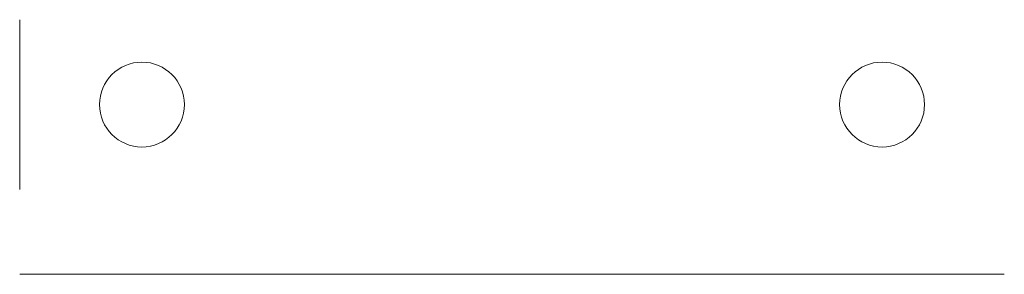
# Model space of a CAD drawing. Units: millimetres. Extents: x 174 to 464, y 0 to 75.
import ezdxf

# ---------------------------------------------------------------- set-up
doc = ezdxf.new("R2010")
doc.units = ezdxf.units.MM
doc.layers.add('M-CONS', color=8, linetype='Continuous', lineweight=13)

msp = doc.modelspace()

# ---------------------------------------------------------------- linework, layer by layer
at = {"layer": 'M-CONS', "extrusion": (0, -1, 0)}
for p, q in [((174.31, 0, -43.65), (464.31, 0, -43.65)), ((174.31, 0, -43.65), (174.31, 0, -13.65)), ((174.31, 0, -13.65), (221.81, 0, -13.65)), ((234.31, 0, -1.15), (234.31, 0, 61.35)), ((259.3, 0, 86.35), (314.31, 0, 86.36)), ((404.19, 0, -1.27), (403.74, 0, 48.82)), ((464.31, 0, -13.65), (416.69, 0, -13.65)), ((464.31, 0, -43.65), (464.31, 0, -13.65))]:
    msp.add_line(p, q, dxfattribs=at)
at = {"layer": 'M-CONS'}
msp.add_polyline3d([(174.31, 25, -13.65), (174.31, 75, -13.65), (174.31, 75, -43.65), (174.31, 25, -43.65)], close=True, dxfattribs=at)
for centre in [(210.31, 50, -13.65), (428.31, 50, -13.65)]:
    msp.add_circle(centre, 12.5, dxfattribs=at)
at = {"layer": 'M-CONS', "extrusion": (0, -1, 0)}
for centre, radius in [((264.31, 55.85), 12.5), ((354.31, 56.35), 50), ((354.31, 56.35), 30)]:
    msp.add_circle(centre, radius, dxfattribs=at)
for centre, radius, start, end in [((221.81, -1.15), 12.5, 270, 0), ((259.31, 61.35), 25, 90.0053, 180), ((416.69, -1.15), 12.5, 180.5226, 270)]:
    msp.add_arc(centre, radius, start, end, dxfattribs=at)

doc.saveas('drawing.dxf')
